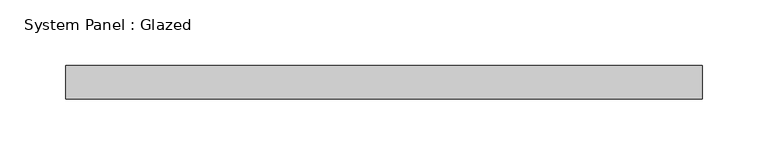
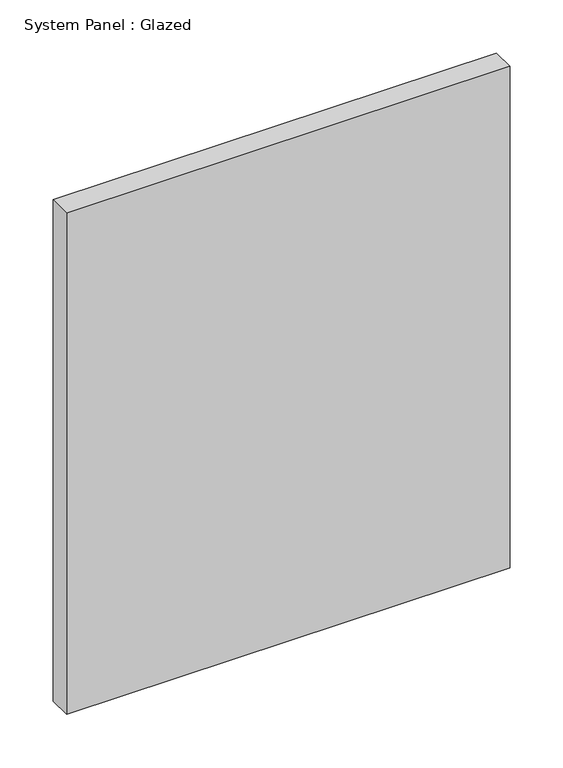
"""IFC4 building model written with IfcOpenShell, lengths in millimetres: plate geometry, System Panel : Glazed."""

from ifc_helpers import new_model, si_unit, origin, origin_with_axes, place, context, project, spatial, polyline, outline, extrude, source, transform, mapped, element, save


def system_panel_glazed_3f46b533(model_context):
    return source(origin(), model_context, "Body", "SweptSolid", [
        extrude(outline(polyline([(241.3, 19.05), (-241.3, 19.05), (-241.3, 44.45), (241.3, 44.45), (241.3, 19.05)])), origin_with_axes(), (0.0, 0.0, 1.0), 576.8647442),
    ])


if __name__ == "__main__":
    model = new_model("IFC4")
    model_context = context("Model", 3, world=origin())
    ifc_project = project(units=[si_unit("LENGTHUNIT", "METRE", prefix="MILLI")], contexts=[model_context])
    site = spatial("IfcSite", under=ifc_project)
    building = spatial("IfcBuilding", under=site)
    placement = place(None, origin())
    system_panel_glazed_shape = system_panel_glazed_3f46b533(model_context)
    element("IfcPlate", 1, ObjectType="System Panel : Glazed", at=placement, inside=building, context=model_context, shape_type="MappedRepresentation", body=[
        mapped(system_panel_glazed_shape, transform((0.0, 0.0, 0.0), x_axis=(1.0, 0.0, 0.0), y_axis=(0.0, 1.0, 0.0), z_axis=(0.0, 0.0, 1.0))),
    ])
    save(model, "model.ifc")

# Revit data of these elements
# Type "System Panel : Glazed"
#   Construction Type Id = "GSP4R"
#   Analytic Construction = "1/8 in Pilkington single glazing"
#   Visual Light Transmittance = 0.9
#   Solar Heat Gain Coefficient = 0.86
#   Heat Transfer Coefficient (U) = 1.18115 BTU/(h·ft²·°F)
#   Define Thermal Properties by = 1
# Element 1 (IfcPlate, "System Panel : Glazed")
#   Materials on its faces: "Glass"
# Materials
#   "Glass": class "Glass", colour RGB 0 128 192, transparency 0.75, Description = "Soda Lime Glass", Cost = 0
